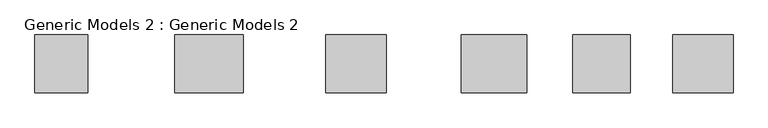
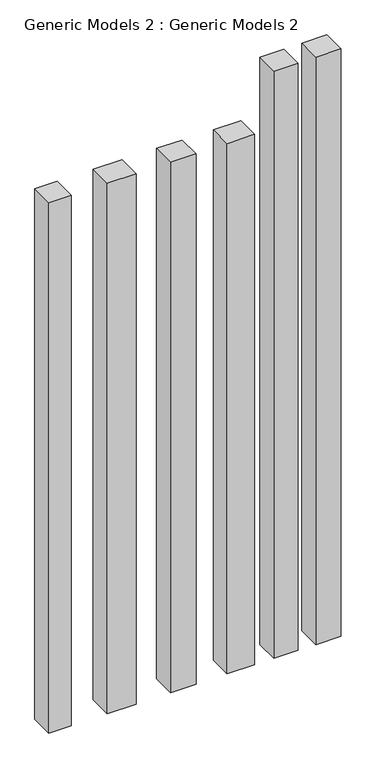
"""IFC4 building model written with IfcOpenShell, lengths in millimetres: proxy geometry, Generic Models 2 : Generic Models 2."""

from ifc_helpers import new_model, si_unit, frame, origin, place, context, project, spatial, polyline, outline, extrude, source, transform, mapped, element, save


def generic_models_2_generic_models_2_c977171b(model_context):
    return source(origin(), model_context, "Body", "SweptSolid", [
        extrude(outline(polyline([(-7994.6824116, -12238.7768247), (-8096.2824116, -12238.7768247), (-8096.2824116, -12137.1768247), (-7994.6824116, -12137.1768247), (-7994.6824116, -12238.7768247)])), frame((0.0, 0.0, 3657.6), z_axis=(0.0, 0.0, 1.0), x_axis=(1.0, 0.0, 0.0)), (0.0, 0.0, 1.0), 2607.2192508),
        extrude(outline(polyline([(-7813.9345733, -12238.7768247), (-7920.0667284, -12238.7768247), (-7920.0667284, -12137.1768247), (-7813.9345733, -12137.1768247), (-7813.9345733, -12238.7768247)])), frame((0.0, 0.0, 3657.6), z_axis=(0.0, 0.0, 1.0), x_axis=(1.0, 0.0, 0.0)), (0.0, 0.0, 1.0), 2607.2192508),
        extrude(outline(polyline([(-8796.4977218, -12238.7768247), (-8796.4977218, -12137.1768247), (-8675.5712442, -12137.1768247), (-8675.5712442, -12238.7768247), (-8796.4977218, -12238.7768247)])), frame((0.0, 0.0, 3657.6), z_axis=(0.0, 0.0, 1.0), x_axis=(1.0, 0.0, 0.0)), (0.0, 0.0, 1.0), 2354.1461963),
        extrude(outline(polyline([(-9042.1407178, -12238.7768247), (-9042.1407178, -12137.1768247), (-8948.787855, -12137.1768247), (-8948.787855, -12238.7768247), (-9042.1407178, -12238.7768247)])), frame((0.0, 0.0, 3657.6), z_axis=(0.0, 0.0, 1.0), x_axis=(1.0, 0.0, 0.0)), (0.0, 0.0, 1.0), 2354.1461963),
        extrude(outline(polyline([(-8424.1536492, -12137.1768247), (-8424.1536492, -12238.7768247), (-8530.942931, -12238.7768247), (-8530.942931, -12137.1768247), (-8424.1536492, -12137.1768247)])), frame((0.0, 0.0, 3657.6), z_axis=(0.0, 0.0, 1.0), x_axis=(1.0, 0.0, 0.0)), (0.0, 0.0, 1.0), 2354.1461963),
        extrude(outline(polyline([(-8176.8750346, -12137.1768247), (-8176.8750346, -12238.7768247), (-8292.2717214, -12238.7768247), (-8292.2717214, -12137.1768247), (-8176.8750346, -12137.1768247)])), frame((0.0, 0.0, 3657.6), z_axis=(0.0, 0.0, 1.0), x_axis=(1.0, 0.0, 0.0)), (0.0, 0.0, 1.0), 2354.1461963),
    ])


if __name__ == "__main__":
    model = new_model("IFC4")
    model_context = context("Model", 3, world=origin())
    ifc_project = project(units=[si_unit("LENGTHUNIT", "METRE", prefix="MILLI")], contexts=[model_context])
    site = spatial("IfcSite", under=ifc_project)
    building = spatial("IfcBuilding", under=site)
    placement = place(None, origin())
    generic_models_2_generic_models_2_shape = generic_models_2_generic_models_2_c977171b(model_context)
    element("IfcBuildingElementProxy", 1, Name="Generic Models 2 : Generic Models 2", ObjectType="Generic Models 2 : Generic Models 2", at=placement, inside=building, context=model_context, shape_type="MappedRepresentation", body=[
        mapped(generic_models_2_generic_models_2_shape, transform((0.0, 0.0, 0.0), x_axis=(1.0, 0.0, 0.0), y_axis=(0.0, 1.0, 0.0), z_axis=(0.0, 0.0, 1.0))),
    ])
    save(model, "model.ifc")
